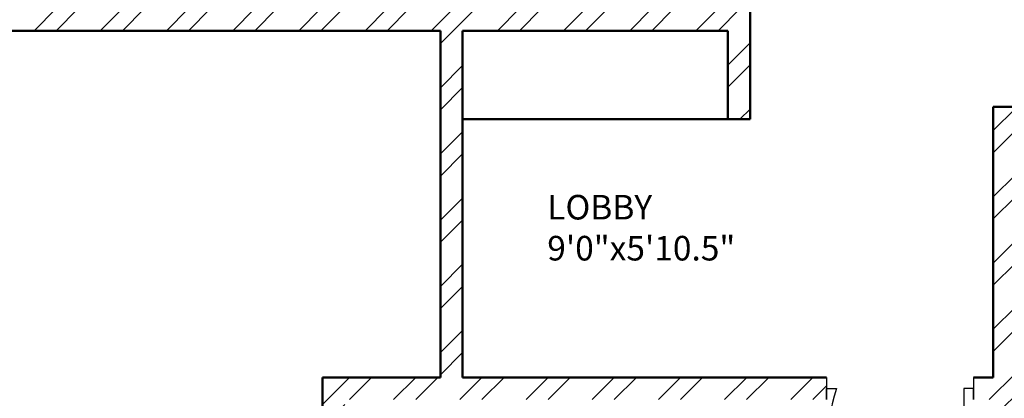
# Model space of a CAD drawing. Units: inches. Extents: x 963 to 2075, y 289 to 2657.
# Tile 28 of 98: x 1310 to 1511, y 1872 to 1949. Entities that reach past the tile are written whole.
import ezdxf

# ---------------------------------------------------------------- set-up
doc = ezdxf.new("R2010")
doc.units = ezdxf.units.IN
for name, color, linetype, lineweight in [('A-AREA-IDEN', 7, 'Continuous', 18), ('A-DOOR', 4, 'Continuous', 25), ('A-WALL', 7, 'Continuous', 50), ('A-WALL-PATT', 8, 'Continuous', 13)]:
    doc.layers.add(name, color=color, linetype=linetype, lineweight=lineweight)
doc.styles.get("Standard").update_dxf_attribs({"font": 'arial.ttf'})

# ---------------------------------------------------------------- blocks, each defined once
blk = doc.blocks.new('DOOR-5')
for p, q in [((0, 38.25), (0, 33.75)), ((29.91, 38.25), (29.91, 33.75)), ((0, 33.75), (0, 36)), ((0, 36), (2, 36)), ((29.91, 36), (27.91, 36)), ((27.91, 36), (27.91, 0)), ((29.91, 33.75), (29.91, 36))]:
    blk.add_line(p, q)
blk.add_arc((27.91, 27.32), 27.32, 161.4794, 270)

msp = doc.modelspace()

# ---------------------------------------------------------------- hatches: boundary and pattern name
at = {"layer": 'A-WALL-PATT'}
h = msp.add_hatch(dxfattribs=at)
h.set_pattern_fill('ANSI32', color=256)
h.paths.add_polyline_path([(1473.61, 2163.07), (1473.61, 2165.32), (1376.42, 2165.32), (1376.42, 2227.98), (1371.92, 2227.98), (1371.92, 2214.82), (1368.41, 2214.82), (1368.41, 2210.32), (1371.92, 2210.32), (1371.92, 2160.82), (1395.92, 2160.82), (1395.92, 2090.32), (1217.34, 2090.32), (1217.34, 2085.82), (1395.92, 2085.82), (1458.92, 2085.82), (1458.92, 2108.32), (1454.42, 2108.32), (1454.42, 2090.32), (1400.42, 2090.32), (1400.42, 2160.82), (1473.61, 2160.82)])
h.paths.add_polyline_path([(1649.42, 2210.32), (1653.23, 2210.32), (1653.23, 2214.82), (1649.42, 2214.82), (1649.42, 2227.98), (1644.92, 2227.98), (1644.92, 2165.32), (1550.1, 2165.32), (1550.1, 2160.82), (1620.92, 2160.82), (1620.92, 2112.82), (1555.45, 2112.82), (1555.45, 2108.32), (1584.33, 2108.32), (1584.33, 2084.92), (1588.83, 2084.92), (1588.83, 2108.32), (1625.42, 2108.32), (1667.95, 2108.32), (1667.95, 2022.67), (1588.83, 2022.67), (1588.83, 2047.41), (1584.33, 2047.41), (1584.33, 1996), (1588.83, 1996), (1588.83, 2018.32), (1667.95, 2018.17), (1667.95, 1928.32), (1625.42, 1928.32), (1625.42, 1923.82), (1672.45, 1923.82), (1672.45, 1928.32), (1672.45, 1946.66), (1785.45, 1946.66), (1785.45, 1951.16), (1743.03, 1951.16), (1743.03, 2017.92), (1841.42, 2017.92), (1841.42, 2014.77), (1845.92, 2014.77), (1845.92, 2017.92), (1905.92, 2017.92), (1905.92, 1987.51), (1910.42, 1987.51), (1910.42, 2022.42), (1910.42, 2068.52), (1905.92, 2068.52), (1905.92, 2022.42), (1845.92, 2022.42), (1845.92, 2025.85), (1843.67, 2025.85), (1841.42, 2025.85), (1841.42, 2022.42), (1743.03, 2022.42), (1743.03, 2084.03), (1768.45, 2084.03), (1785.45, 2084.03), (1785.45, 2088.53), (1672.45, 2088.53), (1672.45, 2112.82), (1667.95, 2112.82), (1625.42, 2112.82), (1625.42, 2160.82), (1649.42, 2160.82)])
h.paths.add_polyline_path([(1672.45, 2084.03), (1738.53, 2084.03), (1738.53, 1951.16), (1672.45, 1951.16)], flags=16)
h.paths.add_polyline_path([(1672.45, 2084.03), (1738.53, 2084.03), (1705.49, 2017.6)], flags=0)
h.paths.add_polyline_path([(1262.77, 2085.82), (1258.27, 2085.82), (1258.27, 2023.28), (1184.42, 2023.28), (1184.42, 2018.78), (1258.27, 2018.78), (1258.27, 1950.82), (1262.77, 1950.82)])
h.paths.add_polyline_path([(1312.27, 2085.82), (1307.77, 2085.82), (1307.77, 1950.82), (1312.27, 1950.82)])
h.paths.add_polyline_path([(1458.92, 1950.82), (1395.92, 1950.82), (1216.57, 1950.82), (1216.57, 1946.32), (1346.42, 1946.32), (1395.92, 1946.32), (1395.92, 1875.82), (1371.92, 1875.82), (1371.92, 1826.32), (1368.93, 1826.32), (1368.93, 1821.82), (1371.92, 1821.82), (1371.92, 1813.62), (1376.42, 1813.62), (1376.42, 1871.32), (1474.5, 1871.32), (1474.5, 1873.57), (1474.5, 1875.82), (1400.42, 1875.82), (1400.42, 1946.32), (1454.42, 1946.32), (1454.42, 1928.32), (1458.92, 1928.32)])
h.paths.add_polyline_path([(1184.42, 2120.78), (1167.92, 2120.78), (1167.92, 2134.81), (1165.67, 2134.81), (1163.42, 2134.81), (1163.42, 2120.78), (1119.92, 2120.78), (1119.92, 2098.1), (1124.42, 2098.1), (1124.42, 2116.28), (1167.92, 2116.28), (1179.92, 2116.28), (1179.92, 2045.92), (1184.42, 2045.92), (1184.42, 2090.32), (1184.42, 2116.28)])
h.paths.add_polyline_path([(1124.42, 2018.78), (1179.92, 2018.78), (1179.92, 2016.29), (1184.42, 2016.29), (1184.42, 2023.28), (1184.42, 2026.59), (1182.17, 2026.59), (1179.92, 2026.59), (1179.92, 2023.28), (1124.42, 2023.28), (1124.42, 2074.1), (1119.92, 2074.1), (1119.92, 2018.78), (1119.92, 1979.63), (1124.42, 1979.63)])
h.paths.add_polyline_path([(1184.42, 1925.78), (1184.42, 1946.32), (1184.42, 1996.07), (1182.17, 1996.07), (1179.92, 1996.07), (1179.92, 1925.78), (1124.42, 1925.78), (1124.42, 1955.63), (1119.92, 1955.5), (1119.92, 1921.28), (1158.92, 1921.28), (1158.92, 1909.98), (1163.42, 1909.98), (1163.42, 1921.28), (1184.42, 1921.28)])
h.paths.add_polyline_path([(1341.45, 1826.32), (1163.42, 1826.32), (1163.42, 1849.98), (1158.92, 1849.98), (1158.92, 1821.82), (1158.92, 1804.03), (1163.42, 1804.03), (1163.42, 1821.82), (1341.45, 1821.82)])
h.paths.add_polyline_path([(1222.98, 1713.82), (1163.42, 1713.82), (1163.42, 1744.03), (1161.17, 1744.03), (1158.92, 1744.03), (1158.92, 1713.82), (1119.92, 1713.82), (1119.92, 1694.65), (1124.42, 1694.65), (1124.42, 1709.32), (1158.92, 1709.32), (1222.98, 1709.32)])
h.paths.add_polyline_path([(1328.42, 1713.82), (1252.04, 1713.82), (1252.04, 1711.57), (1252.04, 1709.32), (1256.42, 1709.32), (1256.42, 1547.32), (1232.94, 1547.32), (1232.94, 1545.07), (1232.94, 1542.82), (1292.42, 1542.82), (1292.42, 1527.63), (1296.92, 1527.63), (1296.92, 1542.82), (1299.46, 1542.82), (1299.46, 1547.32), (1260.92, 1547.32), (1260.92, 1658.32), (1343.66, 1658.32), (1343.66, 1660.57), (1343.66, 1662.82), (1328.42, 1662.82), (1328.42, 1676.59), (1327.4, 1676.59), (1323.92, 1676.59), (1323.92, 1662.82), (1260.92, 1662.82), (1260.92, 1709.32), (1323.92, 1709.32), (1323.92, 1699.85), (1328.42, 1699.85)])
h.paths.add_polyline_path([(1649.42, 1875.82), (1625.42, 1875.82), (1625.42, 1928.32), (1620.92, 1928.32), (1588.83, 1928.32), (1588.83, 1950.59), (1584.33, 1950.59), (1584.33, 1928.32), (1555.45, 1928.32), (1555.45, 1923.82), (1620.92, 1923.82), (1620.92, 1875.82), (1548.95, 1875.82), (1548.95, 1873.57), (1548.95, 1871.32), (1644.92, 1871.32), (1644.92, 1813.62), (1649.42, 1813.62), (1649.42, 1821.82), (1652.04, 1821.82), (1652.04, 1824.07), (1652.04, 1826.32), (1649.42, 1826.32)])
h.paths.add_polyline_path([(1512.92, 1871.32), (1516.48, 1871.32), (1516.48, 1875.82), (1512.92, 1875.82), (1512.92, 1923.82), (1512.92, 1928.32), (1512.92, 1930.83), (1508.42, 1930.83), (1508.42, 1875.82), (1504.41, 1875.82), (1504.41, 1871.32), (1508.42, 1871.32), (1508.42, 1713.82), (1376.42, 1713.82), (1376.42, 1743.32), (1371.92, 1743.32), (1371.92, 1709.32), (1371.92, 1706.01), (1376.42, 1706.01), (1376.42, 1709.32), (1508.42, 1709.32), (1508.42, 1547.32), (1501.87, 1547.32), (1501.87, 1542.82), (1508.42, 1542.82), (1508.42, 1482.82), (1508.42, 1436.32), (1512.92, 1436.32), (1512.92, 1542.82), (1519.32, 1542.82), (1519.32, 1545.07), (1519.32, 1547.32), (1512.92, 1547.32), (1512.92, 1709.32), (1644.92, 1709.32), (1644.92, 1707.55), (1649.42, 1707.55), (1649.42, 1709.32), (1649.42, 1743.32), (1644.92, 1743.32), (1644.92, 1713.82), (1512.92, 1713.82)])
h.paths.add_polyline_path([(1129.88, 1545.07), (1129.88, 1547.32), (1124.42, 1547.32), (1095.92, 1547.32), (1095.92, 1614.82), (1124.42, 1614.82), (1124.42, 1619.32), (1095.92, 1619.32), (1091.42, 1619.32), (1091.42, 1542.82), (1095.92, 1542.82), (1119.92, 1542.82), (1129.88, 1542.82)])
h.paths.add_polyline_path([(1208.42, 1542.82), (1211.74, 1542.82), (1211.74, 1547.32), (1198.85, 1547.32), (1198.85, 1542.82), (1203.92, 1542.82), (1203.92, 1478.32), (1208.42, 1478.32), (1296.92, 1478.32), (1296.92, 1503.63), (1292.42, 1503.63), (1292.42, 1482.82), (1208.42, 1482.82)])
h.paths.add_polyline_path([(1430.42, 1542.82), (1435.7, 1542.82), (1435.7, 1545.07), (1435.7, 1547.32), (1422.66, 1547.32), (1422.66, 1545.07), (1422.66, 1542.82), (1425.92, 1542.82), (1425.92, 1482.86), (1341.92, 1482.86), (1341.92, 1502.73), (1337.42, 1502.73), (1337.42, 1478.36), (1425.92, 1478.36), (1425.92, 1440.82), (1425.92, 1436.32), (1430.42, 1436.32)])
h.paths.add_polyline_path([(1698.48, 2004.26), (1727.69, 2004.26), (1727.69, 2022.92), (1698.48, 2022.92)], flags=8)

# ---------------------------------------------------------------- linework, layer by layer
at = {"layer": 'A-WALL'}
for p, q in [((1458.92, 1950.82), (1458.92, 1928.32)), ((1216.57, 1946.32), (1346.42, 1946.32)), ((1346.42, 1946.32), (1395.92, 1946.32)), ((1395.92, 1946.32), (1346.42, 1946.32)), ((1395.92, 1946.32), (1395.92, 1875.82)), ((1400.42, 1946.32), (1454.42, 1946.32)), ((1400.42, 1875.82), (1400.42, 1946.32)), ((1454.42, 1928.32), (1454.42, 1946.32)), ((1508.42, 1930.83), (1508.42, 1875.82)), ((1508.42, 1930.83), (1512.92, 1930.83)), ((1454.42, 1928.32), (1400.42, 1928.32)), ((1458.92, 1928.32), (1454.42, 1928.32)), ((1371.92, 1875.82), (1371.92, 1826.32)), ((1395.92, 1875.82), (1371.92, 1875.82)), ((1400.42, 1875.82), (1474.5, 1875.82)), ((1504.41, 1875.82), (1508.42, 1875.82))]:
    msp.add_line(p, q, dxfattribs=at)

# ---------------------------------------------------------------- block references
at = {"layer": 'A-DOOR'}
msp.add_blockref('DOOR-5', (1474.5, 1837.57), dxfattribs=at)

# ---------------------------------------------------------------- texts
at = {"layer": 'A-AREA-IDEN', "insert": (1417.65, 1912.93), "char_height": 5, "attachment_point": 1}
msp.add_mtext_dynamic_manual_height_columns('LOBBY\\P9\'0"x5\'10.5"', width=86.1615, gutter_width=12.5, heights=[0], dxfattribs=at)

doc.saveas('drawing.dxf')
